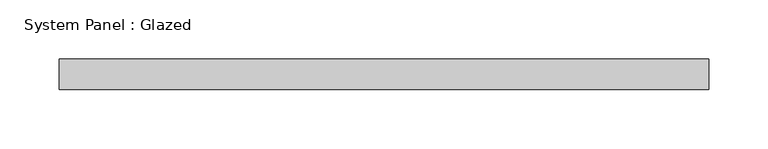
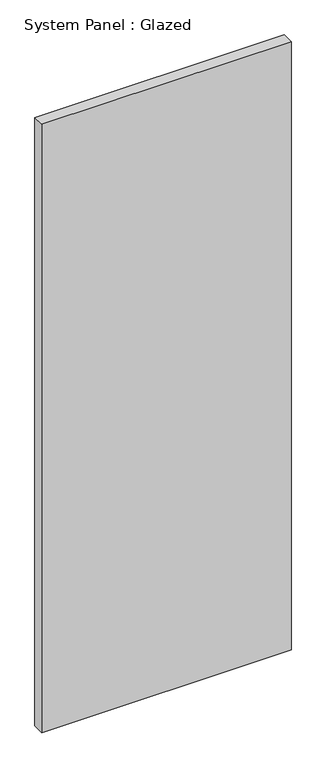
"""IFC4 building model written with IfcOpenShell, lengths in millimetres: plate geometry, System Panel : Glazed."""

from ifc_helpers import new_model, si_unit, origin, origin_with_axes, place, context, project, spatial, polyline, outline, extrude, source, transform, mapped, element, save


def system_panel_glazed_c8fc80f3(model_context):
    return source(origin(), model_context, "Body", "SweptSolid", [
        extrude(outline(polyline([(273.05, 19.05), (-273.05, 19.05), (-273.05, 44.45), (273.05, 44.45), (273.05, 19.05)])), origin_with_axes(), (0.0, 0.0, 1.0), 1409.2264761),
    ])


if __name__ == "__main__":
    model = new_model("IFC4")
    model_context = context("Model", 3, world=origin())
    ifc_project = project(units=[si_unit("LENGTHUNIT", "METRE", prefix="MILLI")], contexts=[model_context])
    site = spatial("IfcSite", under=ifc_project)
    building = spatial("IfcBuilding", under=site)
    placement = place(None, origin())
    system_panel_glazed_shape = system_panel_glazed_c8fc80f3(model_context)
    element("IfcPlate", 1, ObjectType="System Panel : Glazed", at=placement, inside=building, context=model_context, shape_type="MappedRepresentation", body=[
        mapped(system_panel_glazed_shape, transform((0.0, 0.0, 0.0), x_axis=(1.0, 0.0, 0.0), y_axis=(0.0, 1.0, 0.0), z_axis=(0.0, 0.0, 1.0))),
    ])
    save(model, "model.ifc")

# Revit data of these elements
# Type "System Panel : Glazed"
#   Construction Type Id = "GSP4R"
#   Analytic Construction = "1/8 in Pilkington single glazing"
#   Visual Light Transmittance = 0.9
#   Solar Heat Gain Coefficient = 0.86
#   Heat Transfer Coefficient (U) = 1.18115 BTU/(h·ft²·°F)
#   Define Thermal Properties by = 1
# Element 1 (IfcPlate, "System Panel : Glazed")
#   Materials on its faces: "Glass"
# Materials
#   "Glass": class "Glass", colour RGB 0 128 192, transparency 0.75, Description = "Soda Lime Glass", Cost = 0
